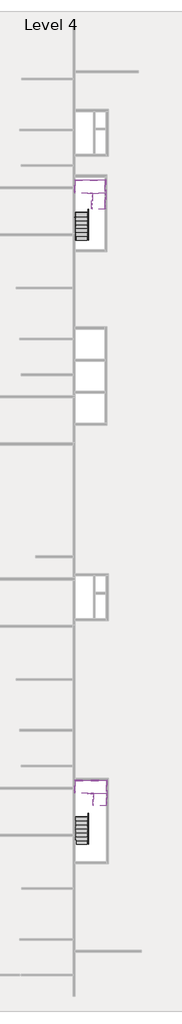
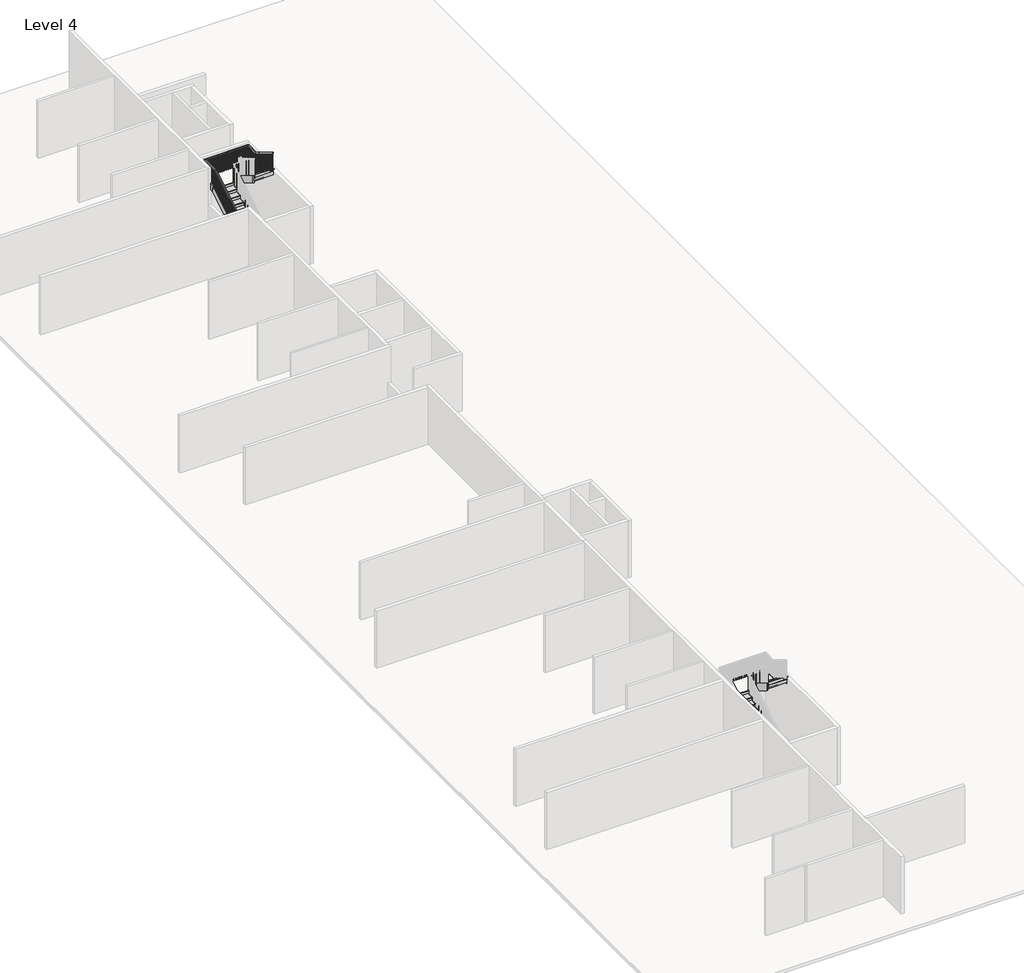
# One storey, part 8 of 8: 16 members, 4 stair flights, 2 slabs, 1 railing.
"""IFC4 building model written with IfcOpenShell, lengths in millimetres."""

from ifc_helpers import new_model, si_unit, frame, origin, place, context, project, spatial, polyline, outline, extrude, faceted_brep, transform, mapped, element, save
from components import non_monolithic_landing_46a25b39, non_monolithic_landing_d45999a6, stair_flight_ca28c9d9, stair_flight_c52ec63c, stair_flight_74cd6fce, stair_flight_e8b6355c

model = new_model("IFC4")

# Units and contexts
model_context = context("Model", 3, world=origin())
ifc_project = project(units=[si_unit("LENGTHUNIT", "METRE", prefix="MILLI")], contexts=[model_context])

# Site, building, storey
site = spatial("IfcSite", under=ifc_project)
building = spatial("IfcBuilding", under=site)
storey = spatial("IfcBuildingStorey", under=building, Name="Level 4", Elevation=34378.6172466)

# Members
placement = place(None, origin())
element("IfcMember", 1, ObjectType="Stringer - 2\" Width", at=placement, inside=storey, context=model_context, shape_type="SweptSolid", body=[
    extrude(outline(polyline([(-23154.3851539, 34378.6172466), (-23154.3851539, 34590.7317586), (-19467.0440987, 36825.4839133), (-19381.8896422, 36520.6839133), (-22916.2996422, 34378.6172466), (-23154.3851539, 34378.6172466)])), frame((-3668.2415084, 0.0, 0.0), z_axis=(1.0, 0.0, 0.0), x_axis=(0.0, 1.0, 0.0)), (0.0, 0.0, 1.0), 50.8),
])
element("IfcMember", 2, ObjectType="Stringer - 2\" Width", at=placement, inside=storey, context=model_context, shape_type="SweptSolid", body=[
    extrude(outline(polyline([(-23154.3851539, 34378.6172466), (-23154.3851539, 34590.7317586), (-19572.9851539, 36761.2772131), (-19572.9851539, 36404.8684516), (-22916.2996422, 34378.6172466), (-23154.3851539, 34378.6172466)])), frame((-2703.0415084, 0.0, 0.0), z_axis=(1.0, 0.0, 0.0), x_axis=(0.0, 1.0, 0.0)), (0.0, 0.0, 1.0), 50.8),
])
element("IfcMember", 3, ObjectType="Stringer - 2\" Width", at=placement, inside=storey, context=model_context, shape_type="SweptSolid", body=[
    extrude(outline(polyline([(-19297.9262092, 36825.4839133), (-19383.0806657, 36520.6839133), (-20360.3851539, 37112.9896637), (-20360.3851539, 37469.3984252), (-19297.9262092, 36825.4839133)])), frame((-1382.2415084, 0.0, 0.0), z_axis=(1.0, 0.0, 0.0), x_axis=(0.0, 1.0, 0.0)), (0.0, 0.0, 1.0), 50.8),
])
element("IfcMember", 4, ObjectType="Stringer - 2\" Width", at=placement, inside=storey, context=model_context, shape_type="SweptSolid", body=[
    extrude(outline(polyline([(-19522.1851539, 36961.3984252), (-19522.1851539, 36604.9896637), (-20360.3851539, 37112.9896637), (-20360.3851539, 37469.3984252), (-19522.1851539, 36961.3984252)])), frame((-2347.4415084, 0.0, 0.0), z_axis=(1.0, 0.0, 0.0), x_axis=(0.0, 1.0, 0.0)), (0.0, 0.0, 1.0), 50.8),
])
element("IfcMember", 5, ObjectType="Stringer - 2\" Width", at=placement, inside=storey, context=model_context, shape_type="Brep", body=[
    faceted_brep([(-1382.2415084, -19297.9262092, 36825.4839133), (-1331.4415084, -19297.9262092, 36825.4839133), (-1331.4415084, -18556.9851539, 36825.4839133), (-1382.2415084, -18607.7851539, 36825.4839133), (-1382.2415084, -19383.0806657, 36520.6839133), (-1382.2415084, -18607.7851539, 36520.6839133), (-1331.4415084, -19383.0806657, 36520.6839133), (-1331.4415084, -18556.9851539, 36520.6839133)], [[[0, 1, 2, 3]], [[4, 0, 3, 5]], [[6, 4, 5, 7]], [[1, 6, 7, 2]], [[1, 0, 4, 6]], [[2, 7, 5, 3]]]),
])
element("IfcMember", 6, ObjectType="Stringer - 2\" Width", at=placement, inside=storey, context=model_context, shape_type="SweptSolid", body=[
    extrude(outline(polyline([(-1331.4415084, -18556.9851539), (-1382.2415084, -18607.7851539), (-3617.4415084, -18607.7851539), (-3668.2415084, -18556.9851539), (-1331.4415084, -18556.9851539)])), frame((0.0, 0.0, 36520.6839133), z_axis=(0.0, 0.0, 1.0), x_axis=(1.0, 0.0, 0.0)), (0.0, 0.0, 1.0), 304.8),
])
element("IfcMember", 7, ObjectType="Stringer - 2\" Width", at=placement, inside=storey, context=model_context, shape_type="Brep", body=[
    faceted_brep([(-3617.4415084, -18607.7851539, 36825.4839133), (-3668.2415084, -18556.9851539, 36825.4839133), (-3668.2415084, -19467.0440987, 36825.4839133), (-3617.4415084, -19467.0440987, 36825.4839133), (-3617.4415084, -18607.7851539, 36520.6839133), (-3617.4415084, -19381.8896422, 36520.6839133), (-3668.2415084, -18556.9851539, 36520.6839133), (-3668.2415084, -19381.8896422, 36520.6839133)], [[[0, 1, 2, 3]], [[4, 0, 3, 5]], [[6, 4, 5, 7]], [[1, 6, 7, 2]], [[1, 0, 4, 6]], [[2, 7, 5, 3]]]),
])
element("IfcMember", 8, ObjectType="Stringer - 2\" Width", at=placement, inside=storey, context=model_context, shape_type="SweptSolid", body=[
    extrude(outline(polyline([(-2703.0415084, -19572.9851539), (-2703.0415084, -19522.1851539), (-2347.4415084, -19522.1851539), (-2347.4415084, -19572.9851539), (-2703.0415084, -19572.9851539)])), frame((0.0, 0.0, 36520.6839133), z_axis=(0.0, 0.0, 1.0), x_axis=(1.0, 0.0, 0.0)), (0.0, 0.0, 1.0), 304.8),
])
element("IfcMember", 9, ObjectType="Stringer - 2\" Width", at=placement, inside=storey, context=model_context, shape_type="SweptSolid", body=[
    extrude(outline(polyline([(19841.9216096, 34378.6172466), (19841.9216096, 34590.7317586), (23249.8626649, 36656.1505799), (23335.0171214, 36351.3505799), (20080.0071214, 34378.6172466), (19841.9216096, 34378.6172466)])), frame((-3668.2415084, 0.0, 0.0), z_axis=(1.0, 0.0, 0.0), x_axis=(0.0, 1.0, 0.0)), (0.0, 0.0, 1.0), 50.8),
])
element("IfcMember", 10, ObjectType="Stringer - 2\" Width", at=placement, inside=storey, context=model_context, shape_type="SweptSolid", body=[
    extrude(outline(polyline([(19841.9216096, 34378.6172466), (19841.9216096, 34590.7317586), (23143.9216096, 36591.9438798), (23143.9216096, 36235.5351183), (20080.0071214, 34378.6172466), (19841.9216096, 34378.6172466)])), frame((-2703.0415084, 0.0, 0.0), z_axis=(1.0, 0.0, 0.0), x_axis=(0.0, 1.0, 0.0)), (0.0, 0.0, 1.0), 50.8),
])
element("IfcMember", 11, ObjectType="Stringer - 2\" Width", at=placement, inside=storey, context=model_context, shape_type="SweptSolid", body=[
    extrude(outline(polyline([(23418.9805543, 36656.1505799), (23333.8260978, 36351.3505799), (22077.1216096, 37112.9896637), (22077.1216096, 37469.3984252), (23418.9805543, 36656.1505799)])), frame((-1483.8415084, 0.0, 0.0), z_axis=(1.0, 0.0, 0.0), x_axis=(0.0, 1.0, 0.0)), (0.0, 0.0, 1.0), 50.8),
])
element("IfcMember", 12, ObjectType="Stringer - 2\" Width", at=placement, inside=storey, context=model_context, shape_type="SweptSolid", body=[
    extrude(outline(polyline([(23194.7216096, 36792.0650919), (23194.7216096, 36435.6563304), (22077.1216096, 37112.9896637), (22077.1216096, 37469.3984252), (23194.7216096, 36792.0650919)])), frame((-2449.0415084, 0.0, 0.0), z_axis=(1.0, 0.0, 0.0), x_axis=(0.0, 1.0, 0.0)), (0.0, 0.0, 1.0), 50.8),
])
element("IfcMember", 13, ObjectType="Stringer - 2\" Width", at=placement, inside=storey, context=model_context, shape_type="Brep", body=[
    faceted_brep([(-1483.8415084, 23418.9805543, 36656.1505799), (-1433.0415084, 23418.9805543, 36656.1505799), (-1433.0415084, 24159.9216096, 36656.1505799), (-1483.8415084, 24109.1216096, 36656.1505799), (-1483.8415084, 23333.8260978, 36351.3505799), (-1483.8415084, 24109.1216096, 36351.3505799), (-1433.0415084, 23333.8260978, 36351.3505799), (-1433.0415084, 24159.9216096, 36351.3505799)], [[[0, 1, 2, 3]], [[4, 0, 3, 5]], [[6, 4, 5, 7]], [[1, 6, 7, 2]], [[1, 0, 4, 6]], [[2, 7, 5, 3]]]),
])
element("IfcMember", 14, ObjectType="Stringer - 2\" Width", at=placement, inside=storey, context=model_context, shape_type="SweptSolid", body=[
    extrude(outline(polyline([(-1433.0415084, 24159.9216096), (-1483.8415084, 24109.1216096), (-3617.4415084, 24109.1216096), (-3668.2415084, 24159.9216096), (-1433.0415084, 24159.9216096)])), frame((0.0, 0.0, 36351.3505799), z_axis=(0.0, 0.0, 1.0), x_axis=(1.0, 0.0, 0.0)), (0.0, 0.0, 1.0), 304.8),
])
element("IfcMember", 15, ObjectType="Stringer - 2\" Width", at=placement, inside=storey, context=model_context, shape_type="Brep", body=[
    faceted_brep([(-3617.4415084, 24109.1216096, 36656.1505799), (-3668.2415084, 24159.9216096, 36656.1505799), (-3668.2415084, 23249.8626649, 36656.1505799), (-3617.4415084, 23249.8626649, 36656.1505799), (-3617.4415084, 24109.1216096, 36351.3505799), (-3617.4415084, 23335.0171214, 36351.3505799), (-3668.2415084, 24159.9216096, 36351.3505799), (-3668.2415084, 23335.0171214, 36351.3505799)], [[[0, 1, 2, 3]], [[4, 0, 3, 5]], [[6, 4, 5, 7]], [[1, 6, 7, 2]], [[1, 0, 4, 6]], [[2, 7, 5, 3]]]),
])
element("IfcMember", 16, ObjectType="Stringer - 2\" Width", at=placement, inside=storey, context=model_context, shape_type="SweptSolid", body=[
    extrude(outline(polyline([(-2703.0415084, 23143.9216096), (-2703.0415084, 23194.7216096), (-2449.0415084, 23194.7216096), (-2449.0415084, 23143.9216096), (-2703.0415084, 23143.9216096)])), frame((0.0, 0.0, 36351.3505799), z_axis=(0.0, 0.0, 1.0), x_axis=(1.0, 0.0, 0.0)), (0.0, 0.0, 1.0), 304.8),
])

# Railing
element("IfcRailing", 17, ObjectType="Handrail - Rectangular", at=placement, inside=storey, context=model_context, shape_type="SolidModel", body=[
    faceted_brep([(-3617.4415084, 19841.9216096, 35462.3505799), (-3617.4415084, 19841.9216096, 35402.9491197), (-3566.6415084, 19841.9216096, 35402.9491197), (-3566.6415084, 19841.9216096, 35462.3505799), (-3617.4415084, 23194.7216096, 37494.3505799), (-3617.4415084, 23208.914019, 37443.5505799), (-3566.6415084, 23208.914019, 37443.5505799), (-3566.6415084, 23194.7216096, 37494.3505799), (-3617.4415084, 24109.1216096, 37494.3505799), (-3617.4415084, 24109.1216096, 37443.5505799), (-3566.6415084, 24058.3216096, 37443.5505799), (-3566.6415084, 24058.3216096, 37494.3505799), (-1483.8415084, 24109.1216096, 37494.3505799), (-1483.8415084, 24109.1216096, 37443.5505799), (-1534.6415084, 24058.3216096, 37443.5505799), (-1534.6415084, 24058.3216096, 37494.3505799), (-1483.8415084, 23474.1216096, 37494.3505799), (-1483.8415084, 23459.9292002, 37443.5505799), (-1534.6415084, 23459.9292002, 37443.5505799), (-1534.6415084, 23474.1216096, 37494.3505799), (-1483.8415084, 23194.7216096, 37663.6839133), (-1483.8415084, 23168.3918824, 37620.2398634), (-1534.6415084, 23168.3918824, 37620.2398634), (-1534.6415084, 23194.7216096, 37663.6839133), (-1483.8415084, 22077.1216096, 38341.0172466), (-1534.6415084, 22077.1216096, 38341.0172466), (-1534.6415084, 22077.1216096, 38281.6157863), (-1483.8415084, 22077.1216096, 38281.6157863)], [[[0, 1, 2, 3]], [[1, 0, 4, 5]], [[2, 1, 5, 6]], [[3, 2, 6, 7]], [[0, 3, 7, 4]], [[5, 4, 8, 9]], [[6, 5, 9, 10]], [[7, 6, 10, 11]], [[4, 7, 11, 8]], [[9, 8, 12, 13]], [[10, 9, 13, 14]], [[11, 10, 14, 15]], [[8, 11, 15, 12]], [[13, 12, 16, 17]], [[14, 13, 17, 18]], [[15, 14, 18, 19]], [[12, 15, 19, 16]], [[17, 16, 20, 21]], [[18, 17, 21, 22]], [[19, 18, 22, 23]], [[16, 19, 23, 20]], [[24, 25, 26, 27]], [[21, 20, 24, 27]], [[22, 21, 27, 26]], [[23, 22, 26, 25]], [[20, 23, 25, 24]]]),
    extrude(outline(polyline([(22188.2466096, 38214.2673015), (22188.2466096, 37257.2839133), (22169.1966096, 37257.2839133), (22169.1966096, 38225.812756), (22188.2466096, 38214.2673015)])), frame((-1518.7665084, 0.0, 0.0), z_axis=(1.0, 0.0, 0.0), x_axis=(0.0, 1.0, 0.0)), (0.0, 0.0, 1.0), 19.05),
    extrude(outline(polyline([(22289.8466096, 38152.6915439), (22289.8466096, 37257.2839133), (22270.7966096, 37257.2839133), (22270.7966096, 38164.2369985), (22289.8466096, 38152.6915439)])), frame((-1518.7665084, 0.0, 0.0), z_axis=(1.0, 0.0, 0.0), x_axis=(0.0, 1.0, 0.0)), (0.0, 0.0, 1.0), 19.05),
    extrude(outline(polyline([(22391.4466096, 38091.1157863), (22391.4466096, 37087.9505799), (22372.3966096, 37087.9505799), (22372.3966096, 38102.6612409), (22391.4466096, 38091.1157863)])), frame((-1518.7665084, 0.0, 0.0), z_axis=(1.0, 0.0, 0.0), x_axis=(0.0, 1.0, 0.0)), (0.0, 0.0, 1.0), 19.05),
    extrude(outline(polyline([(22493.0466096, 38029.5400288), (22493.0466096, 37087.9505799), (22473.9966096, 37087.9505799), (22473.9966096, 38041.0854833), (22493.0466096, 38029.5400288)])), frame((-1518.7665084, 0.0, 0.0), z_axis=(1.0, 0.0, 0.0), x_axis=(0.0, 1.0, 0.0)), (0.0, 0.0, 1.0), 19.05),
    extrude(outline(polyline([(22594.6466096, 37967.9642712), (22594.6466096, 37087.9505799), (22575.5966096, 37087.9505799), (22575.5966096, 37979.5097257), (22594.6466096, 37967.9642712)])), frame((-1518.7665084, 0.0, 0.0), z_axis=(1.0, 0.0, 0.0), x_axis=(0.0, 1.0, 0.0)), (0.0, 0.0, 1.0), 19.05),
    extrude(outline(polyline([(22696.2466096, 37906.3885136), (22696.2466096, 36918.6172466), (22677.1966096, 36918.6172466), (22677.1966096, 37917.9339682), (22696.2466096, 37906.3885136)])), frame((-1518.7665084, 0.0, 0.0), z_axis=(1.0, 0.0, 0.0), x_axis=(0.0, 1.0, 0.0)), (0.0, 0.0, 1.0), 19.05),
    extrude(outline(polyline([(22797.8466096, 37844.812756), (22797.8466096, 36918.6172466), (22778.7966096, 36918.6172466), (22778.7966096, 37856.3582106), (22797.8466096, 37844.812756)])), frame((-1518.7665084, 0.0, 0.0), z_axis=(1.0, 0.0, 0.0), x_axis=(0.0, 1.0, 0.0)), (0.0, 0.0, 1.0), 19.05),
    extrude(outline(polyline([(22899.4466096, 37783.2369985), (22899.4466096, 36918.6172466), (22880.3966096, 36918.6172466), (22880.3966096, 37794.782453), (22899.4466096, 37783.2369985)])), frame((-1518.7665084, 0.0, 0.0), z_axis=(1.0, 0.0, 0.0), x_axis=(0.0, 1.0, 0.0)), (0.0, 0.0, 1.0), 19.05),
    extrude(outline(polyline([(23001.0466096, 37721.6612409), (23001.0466096, 36749.2839133), (22981.9966096, 36749.2839133), (22981.9966096, 37733.2066954), (23001.0466096, 37721.6612409)])), frame((-1518.7665084, 0.0, 0.0), z_axis=(1.0, 0.0, 0.0), x_axis=(0.0, 1.0, 0.0)), (0.0, 0.0, 1.0), 19.05),
    extrude(outline(polyline([(23102.6466096, 37660.0854833), (23102.6466096, 36749.2839133), (23083.5966096, 36749.2839133), (23083.5966096, 37671.6309379), (23102.6466096, 37660.0854833)])), frame((-1518.7665084, 0.0, 0.0), z_axis=(1.0, 0.0, 0.0), x_axis=(0.0, 1.0, 0.0)), (0.0, 0.0, 1.0), 19.05),
    extrude(outline(polyline([(23280.4466096, 37552.3279076), (23280.4466096, 36579.9505799), (23261.3966096, 36579.9505799), (23261.3966096, 37563.8733621), (23280.4466096, 37552.3279076)])), frame((-1518.7665084, 0.0, 0.0), z_axis=(1.0, 0.0, 0.0), x_axis=(0.0, 1.0, 0.0)), (0.0, 0.0, 1.0), 19.05),
    extrude(outline(polyline([(23382.0466096, 37490.75215), (23382.0466096, 36579.9505799), (23362.9966096, 36579.9505799), (23362.9966096, 37502.2976045), (23382.0466096, 37490.75215)])), frame((-1518.7665084, 0.0, 0.0), z_axis=(1.0, 0.0, 0.0), x_axis=(0.0, 1.0, 0.0)), (0.0, 0.0, 1.0), 19.05),
    extrude(outline(polyline([(-1499.7165084, 23483.6466096), (-1499.7165084, 23464.5966096), (-1518.7665084, 23464.5966096), (-1518.7665084, 23483.6466096), (-1499.7165084, 23483.6466096)])), frame((0.0, 0.0, 36579.9505799), z_axis=(0.0, 0.0, 1.0), x_axis=(1.0, 0.0, 0.0)), (0.0, 0.0, 1.0), 863.6),
    extrude(outline(polyline([(-1499.7165084, 23585.2466096), (-1499.7165084, 23566.1966096), (-1518.7665084, 23566.1966096), (-1518.7665084, 23585.2466096), (-1499.7165084, 23585.2466096)])), frame((0.0, 0.0, 36579.9505799), z_axis=(0.0, 0.0, 1.0), x_axis=(1.0, 0.0, 0.0)), (0.0, 0.0, 1.0), 863.6),
    extrude(outline(polyline([(-1499.7165084, 23686.8466096), (-1499.7165084, 23667.7966096), (-1518.7665084, 23667.7966096), (-1518.7665084, 23686.8466096), (-1499.7165084, 23686.8466096)])), frame((0.0, 0.0, 36579.9505799), z_axis=(0.0, 0.0, 1.0), x_axis=(1.0, 0.0, 0.0)), (0.0, 0.0, 1.0), 863.6),
    extrude(outline(polyline([(-1499.7165084, 23788.4466096), (-1499.7165084, 23769.3966096), (-1518.7665084, 23769.3966096), (-1518.7665084, 23788.4466096), (-1499.7165084, 23788.4466096)])), frame((0.0, 0.0, 36579.9505799), z_axis=(0.0, 0.0, 1.0), x_axis=(1.0, 0.0, 0.0)), (0.0, 0.0, 1.0), 863.6),
    extrude(outline(polyline([(-1499.7165084, 23890.0466096), (-1499.7165084, 23870.9966096), (-1518.7665084, 23870.9966096), (-1518.7665084, 23890.0466096), (-1499.7165084, 23890.0466096)])), frame((0.0, 0.0, 36579.9505799), z_axis=(0.0, 0.0, 1.0), x_axis=(1.0, 0.0, 0.0)), (0.0, 0.0, 1.0), 863.6),
    extrude(outline(polyline([(-1499.7165084, 23991.6466096), (-1499.7165084, 23972.5966096), (-1518.7665084, 23972.5966096), (-1518.7665084, 23991.6466096), (-1499.7165084, 23991.6466096)])), frame((0.0, 0.0, 36579.9505799), z_axis=(0.0, 0.0, 1.0), x_axis=(1.0, 0.0, 0.0)), (0.0, 0.0, 1.0), 863.6),
    extrude(outline(polyline([(-1569.5665084, 24093.2466096), (-1550.5165084, 24093.2466096), (-1550.5165084, 24074.1966096), (-1569.5665084, 24074.1966096), (-1569.5665084, 24093.2466096)])), frame((0.0, 0.0, 36579.9505799), z_axis=(0.0, 0.0, 1.0), x_axis=(1.0, 0.0, 0.0)), (0.0, 0.0, 1.0), 863.6),
    extrude(outline(polyline([(-1671.1665084, 24093.2466096), (-1652.1165084, 24093.2466096), (-1652.1165084, 24074.1966096), (-1671.1665084, 24074.1966096), (-1671.1665084, 24093.2466096)])), frame((0.0, 0.0, 36579.9505799), z_axis=(0.0, 0.0, 1.0), x_axis=(1.0, 0.0, 0.0)), (0.0, 0.0, 1.0), 863.6),
    extrude(outline(polyline([(-1772.7665084, 24093.2466096), (-1753.7165084, 24093.2466096), (-1753.7165084, 24074.1966096), (-1772.7665084, 24074.1966096), (-1772.7665084, 24093.2466096)])), frame((0.0, 0.0, 36579.9505799), z_axis=(0.0, 0.0, 1.0), x_axis=(1.0, 0.0, 0.0)), (0.0, 0.0, 1.0), 863.6),
    extrude(outline(polyline([(-1874.3665084, 24093.2466096), (-1855.3165084, 24093.2466096), (-1855.3165084, 24074.1966096), (-1874.3665084, 24074.1966096), (-1874.3665084, 24093.2466096)])), frame((0.0, 0.0, 36579.9505799), z_axis=(0.0, 0.0, 1.0), x_axis=(1.0, 0.0, 0.0)), (0.0, 0.0, 1.0), 863.6),
    extrude(outline(polyline([(-1975.9665084, 24093.2466096), (-1956.9165084, 24093.2466096), (-1956.9165084, 24074.1966096), (-1975.9665084, 24074.1966096), (-1975.9665084, 24093.2466096)])), frame((0.0, 0.0, 36579.9505799), z_axis=(0.0, 0.0, 1.0), x_axis=(1.0, 0.0, 0.0)), (0.0, 0.0, 1.0), 863.6),
    extrude(outline(polyline([(-2077.5665084, 24093.2466096), (-2058.5165084, 24093.2466096), (-2058.5165084, 24074.1966096), (-2077.5665084, 24074.1966096), (-2077.5665084, 24093.2466096)])), frame((0.0, 0.0, 36579.9505799), z_axis=(0.0, 0.0, 1.0), x_axis=(1.0, 0.0, 0.0)), (0.0, 0.0, 1.0), 863.6),
    extrude(outline(polyline([(-2179.1665084, 24093.2466096), (-2160.1165084, 24093.2466096), (-2160.1165084, 24074.1966096), (-2179.1665084, 24074.1966096), (-2179.1665084, 24093.2466096)])), frame((0.0, 0.0, 36579.9505799), z_axis=(0.0, 0.0, 1.0), x_axis=(1.0, 0.0, 0.0)), (0.0, 0.0, 1.0), 863.6),
    extrude(outline(polyline([(-2280.7665084, 24093.2466096), (-2261.7165084, 24093.2466096), (-2261.7165084, 24074.1966096), (-2280.7665084, 24074.1966096), (-2280.7665084, 24093.2466096)])), frame((0.0, 0.0, 36579.9505799), z_axis=(0.0, 0.0, 1.0), x_axis=(1.0, 0.0, 0.0)), (0.0, 0.0, 1.0), 863.6),
    extrude(outline(polyline([(-2382.3665084, 24093.2466096), (-2363.3165084, 24093.2466096), (-2363.3165084, 24074.1966096), (-2382.3665084, 24074.1966096), (-2382.3665084, 24093.2466096)])), frame((0.0, 0.0, 36579.9505799), z_axis=(0.0, 0.0, 1.0), x_axis=(1.0, 0.0, 0.0)), (0.0, 0.0, 1.0), 863.6),
    extrude(outline(polyline([(-2483.9665084, 24093.2466096), (-2464.9165084, 24093.2466096), (-2464.9165084, 24074.1966096), (-2483.9665084, 24074.1966096), (-2483.9665084, 24093.2466096)])), frame((0.0, 0.0, 36579.9505799), z_axis=(0.0, 0.0, 1.0), x_axis=(1.0, 0.0, 0.0)), (0.0, 0.0, 1.0), 863.6),
    extrude(outline(polyline([(-2585.5665084, 24093.2466096), (-2566.5165084, 24093.2466096), (-2566.5165084, 24074.1966096), (-2585.5665084, 24074.1966096), (-2585.5665084, 24093.2466096)])), frame((0.0, 0.0, 36579.9505799), z_axis=(0.0, 0.0, 1.0), x_axis=(1.0, 0.0, 0.0)), (0.0, 0.0, 1.0), 863.6),
    extrude(outline(polyline([(-2687.1665084, 24093.2466096), (-2668.1165084, 24093.2466096), (-2668.1165084, 24074.1966096), (-2687.1665084, 24074.1966096), (-2687.1665084, 24093.2466096)])), frame((0.0, 0.0, 36579.9505799), z_axis=(0.0, 0.0, 1.0), x_axis=(1.0, 0.0, 0.0)), (0.0, 0.0, 1.0), 863.6),
    extrude(outline(polyline([(-2788.7665084, 24093.2466096), (-2769.7165084, 24093.2466096), (-2769.7165084, 24074.1966096), (-2788.7665084, 24074.1966096), (-2788.7665084, 24093.2466096)])), frame((0.0, 0.0, 36579.9505799), z_axis=(0.0, 0.0, 1.0), x_axis=(1.0, 0.0, 0.0)), (0.0, 0.0, 1.0), 863.6),
    extrude(outline(polyline([(-2890.3665084, 24093.2466096), (-2871.3165084, 24093.2466096), (-2871.3165084, 24074.1966096), (-2890.3665084, 24074.1966096), (-2890.3665084, 24093.2466096)])), frame((0.0, 0.0, 36579.9505799), z_axis=(0.0, 0.0, 1.0), x_axis=(1.0, 0.0, 0.0)), (0.0, 0.0, 1.0), 863.6),
    extrude(outline(polyline([(-2991.9665084, 24093.2466096), (-2972.9165084, 24093.2466096), (-2972.9165084, 24074.1966096), (-2991.9665084, 24074.1966096), (-2991.9665084, 24093.2466096)])), frame((0.0, 0.0, 36579.9505799), z_axis=(0.0, 0.0, 1.0), x_axis=(1.0, 0.0, 0.0)), (0.0, 0.0, 1.0), 863.6),
    extrude(outline(polyline([(-3093.5665084, 24093.2466096), (-3074.5165084, 24093.2466096), (-3074.5165084, 24074.1966096), (-3093.5665084, 24074.1966096), (-3093.5665084, 24093.2466096)])), frame((0.0, 0.0, 36579.9505799), z_axis=(0.0, 0.0, 1.0), x_axis=(1.0, 0.0, 0.0)), (0.0, 0.0, 1.0), 863.6),
    extrude(outline(polyline([(-3195.1665084, 24093.2466096), (-3176.1165084, 24093.2466096), (-3176.1165084, 24074.1966096), (-3195.1665084, 24074.1966096), (-3195.1665084, 24093.2466096)])), frame((0.0, 0.0, 36579.9505799), z_axis=(0.0, 0.0, 1.0), x_axis=(1.0, 0.0, 0.0)), (0.0, 0.0, 1.0), 863.6),
    extrude(outline(polyline([(-3296.7665084, 24093.2466096), (-3277.7165084, 24093.2466096), (-3277.7165084, 24074.1966096), (-3296.7665084, 24074.1966096), (-3296.7665084, 24093.2466096)])), frame((0.0, 0.0, 36579.9505799), z_axis=(0.0, 0.0, 1.0), x_axis=(1.0, 0.0, 0.0)), (0.0, 0.0, 1.0), 863.6),
    extrude(outline(polyline([(-3398.3665084, 24093.2466096), (-3379.3165084, 24093.2466096), (-3379.3165084, 24074.1966096), (-3398.3665084, 24074.1966096), (-3398.3665084, 24093.2466096)])), frame((0.0, 0.0, 36579.9505799), z_axis=(0.0, 0.0, 1.0), x_axis=(1.0, 0.0, 0.0)), (0.0, 0.0, 1.0), 863.6),
    extrude(outline(polyline([(-3499.9665084, 24093.2466096), (-3480.9165084, 24093.2466096), (-3480.9165084, 24074.1966096), (-3499.9665084, 24074.1966096), (-3499.9665084, 24093.2466096)])), frame((0.0, 0.0, 36579.9505799), z_axis=(0.0, 0.0, 1.0), x_axis=(1.0, 0.0, 0.0)), (0.0, 0.0, 1.0), 863.6),
    extrude(outline(polyline([(-3601.5665084, 23997.9966096), (-3601.5665084, 24017.0466096), (-3582.5165084, 24017.0466096), (-3582.5165084, 23997.9966096), (-3601.5665084, 23997.9966096)])), frame((0.0, 0.0, 36579.9505799), z_axis=(0.0, 0.0, 1.0), x_axis=(1.0, 0.0, 0.0)), (0.0, 0.0, 1.0), 863.6),
    extrude(outline(polyline([(-3601.5665084, 23896.3966096), (-3601.5665084, 23915.4466096), (-3582.5165084, 23915.4466096), (-3582.5165084, 23896.3966096), (-3601.5665084, 23896.3966096)])), frame((0.0, 0.0, 36579.9505799), z_axis=(0.0, 0.0, 1.0), x_axis=(1.0, 0.0, 0.0)), (0.0, 0.0, 1.0), 863.6),
    extrude(outline(polyline([(-3601.5665084, 23794.7966096), (-3601.5665084, 23813.8466096), (-3582.5165084, 23813.8466096), (-3582.5165084, 23794.7966096), (-3601.5665084, 23794.7966096)])), frame((0.0, 0.0, 36579.9505799), z_axis=(0.0, 0.0, 1.0), x_axis=(1.0, 0.0, 0.0)), (0.0, 0.0, 1.0), 863.6),
    extrude(outline(polyline([(-3601.5665084, 23693.1966096), (-3601.5665084, 23712.2466096), (-3582.5165084, 23712.2466096), (-3582.5165084, 23693.1966096), (-3601.5665084, 23693.1966096)])), frame((0.0, 0.0, 36579.9505799), z_axis=(0.0, 0.0, 1.0), x_axis=(1.0, 0.0, 0.0)), (0.0, 0.0, 1.0), 863.6),
    extrude(outline(polyline([(-3601.5665084, 23591.5966096), (-3601.5665084, 23610.6466096), (-3582.5165084, 23610.6466096), (-3582.5165084, 23591.5966096), (-3601.5665084, 23591.5966096)])), frame((0.0, 0.0, 36579.9505799), z_axis=(0.0, 0.0, 1.0), x_axis=(1.0, 0.0, 0.0)), (0.0, 0.0, 1.0), 863.6),
    extrude(outline(polyline([(-3601.5665084, 23489.9966096), (-3601.5665084, 23509.0466096), (-3582.5165084, 23509.0466096), (-3582.5165084, 23489.9966096), (-3601.5665084, 23489.9966096)])), frame((0.0, 0.0, 36579.9505799), z_axis=(0.0, 0.0, 1.0), x_axis=(1.0, 0.0, 0.0)), (0.0, 0.0, 1.0), 863.6),
    extrude(outline(polyline([(-3601.5665084, 23388.3966096), (-3601.5665084, 23407.4466096), (-3582.5165084, 23407.4466096), (-3582.5165084, 23388.3966096), (-3601.5665084, 23388.3966096)])), frame((0.0, 0.0, 36579.9505799), z_axis=(0.0, 0.0, 1.0), x_axis=(1.0, 0.0, 0.0)), (0.0, 0.0, 1.0), 863.6),
    extrude(outline(polyline([(-3601.5665084, 23286.7966096), (-3601.5665084, 23305.8466096), (-3582.5165084, 23305.8466096), (-3582.5165084, 23286.7966096), (-3601.5665084, 23286.7966096)])), frame((0.0, 0.0, 36579.9505799), z_axis=(0.0, 0.0, 1.0), x_axis=(1.0, 0.0, 0.0)), (0.0, 0.0, 1.0), 863.6),
    extrude(outline(polyline([(23102.6466096, 37379.1460894), (23102.6466096, 36410.6172466), (23083.5966096, 36410.6172466), (23083.5966096, 37367.6006348), (23102.6466096, 37379.1460894)])), frame((-3601.5665084, 0.0, 0.0), z_axis=(1.0, 0.0, 0.0), x_axis=(0.0, 1.0, 0.0)), (0.0, 0.0, 1.0), 19.05),
    extrude(outline(polyline([(23001.0466096, 37317.5703318), (23001.0466096, 36410.6172466), (22981.9966096, 36410.6172466), (22981.9966096, 37306.0248773), (23001.0466096, 37317.5703318)])), frame((-3601.5665084, 0.0, 0.0), z_axis=(1.0, 0.0, 0.0), x_axis=(0.0, 1.0, 0.0)), (0.0, 0.0, 1.0), 19.05),
    extrude(outline(polyline([(22899.4466096, 37255.9945742), (22899.4466096, 36241.2839133), (22880.3966096, 36241.2839133), (22880.3966096, 37244.4491197), (22899.4466096, 37255.9945742)])), frame((-3601.5665084, 0.0, 0.0), z_axis=(1.0, 0.0, 0.0), x_axis=(0.0, 1.0, 0.0)), (0.0, 0.0, 1.0), 19.05),
    extrude(outline(polyline([(22797.8466096, 37194.4188166), (22797.8466096, 36241.2839133), (22778.7966096, 36241.2839133), (22778.7966096, 37182.8733621), (22797.8466096, 37194.4188166)])), frame((-3601.5665084, 0.0, 0.0), z_axis=(1.0, 0.0, 0.0), x_axis=(0.0, 1.0, 0.0)), (0.0, 0.0, 1.0), 19.05),
    extrude(outline(polyline([(22696.2466096, 37132.8430591), (22696.2466096, 36241.2839133), (22677.1966096, 36241.2839133), (22677.1966096, 37121.2976045), (22696.2466096, 37132.8430591)])), frame((-3601.5665084, 0.0, 0.0), z_axis=(1.0, 0.0, 0.0), x_axis=(0.0, 1.0, 0.0)), (0.0, 0.0, 1.0), 19.05),
    extrude(outline(polyline([(22594.6466096, 37071.2673015), (22594.6466096, 36071.9505799), (22575.5966096, 36071.9505799), (22575.5966096, 37059.721847), (22594.6466096, 37071.2673015)])), frame((-3601.5665084, 0.0, 0.0), z_axis=(1.0, 0.0, 0.0), x_axis=(0.0, 1.0, 0.0)), (0.0, 0.0, 1.0), 19.05),
    extrude(outline(polyline([(22493.0466096, 37009.6915439), (22493.0466096, 36071.9505799), (22473.9966096, 36071.9505799), (22473.9966096, 36998.1460894), (22493.0466096, 37009.6915439)])), frame((-3601.5665084, 0.0, 0.0), z_axis=(1.0, 0.0, 0.0), x_axis=(0.0, 1.0, 0.0)), (0.0, 0.0, 1.0), 19.05),
    extrude(outline(polyline([(22391.4466096, 36948.1157863), (22391.4466096, 36071.9505799), (22372.3966096, 36071.9505799), (22372.3966096, 36936.5703318), (22391.4466096, 36948.1157863)])), frame((-3601.5665084, 0.0, 0.0), z_axis=(1.0, 0.0, 0.0), x_axis=(0.0, 1.0, 0.0)), (0.0, 0.0, 1.0), 19.05),
    extrude(outline(polyline([(22289.8466096, 36886.5400288), (22289.8466096, 35902.6172466), (22270.7966096, 35902.6172466), (22270.7966096, 36874.9945742), (22289.8466096, 36886.5400288)])), frame((-3601.5665084, 0.0, 0.0), z_axis=(1.0, 0.0, 0.0), x_axis=(0.0, 1.0, 0.0)), (0.0, 0.0, 1.0), 19.05),
    extrude(outline(polyline([(22188.2466096, 36824.9642712), (22188.2466096, 35902.6172466), (22169.1966096, 35902.6172466), (22169.1966096, 36813.4188166), (22188.2466096, 36824.9642712)])), frame((-3601.5665084, 0.0, 0.0), z_axis=(1.0, 0.0, 0.0), x_axis=(0.0, 1.0, 0.0)), (0.0, 0.0, 1.0), 19.05),
    extrude(outline(polyline([(22086.6466096, 36763.3885136), (22086.6466096, 35902.6172466), (22067.5966096, 35902.6172466), (22067.5966096, 36751.8430591), (22086.6466096, 36763.3885136)])), frame((-3601.5665084, 0.0, 0.0), z_axis=(1.0, 0.0, 0.0), x_axis=(0.0, 1.0, 0.0)), (0.0, 0.0, 1.0), 19.05),
    extrude(outline(polyline([(21985.0466096, 36701.812756), (21985.0466096, 35733.2839133), (21965.9966096, 35733.2839133), (21965.9966096, 36690.2673015), (21985.0466096, 36701.812756)])), frame((-3601.5665084, 0.0, 0.0), z_axis=(1.0, 0.0, 0.0), x_axis=(0.0, 1.0, 0.0)), (0.0, 0.0, 1.0), 19.05),
    extrude(outline(polyline([(21883.4466096, 36640.2369985), (21883.4466096, 35733.2839133), (21864.3966096, 35733.2839133), (21864.3966096, 36628.6915439), (21883.4466096, 36640.2369985)])), frame((-3601.5665084, 0.0, 0.0), z_axis=(1.0, 0.0, 0.0), x_axis=(0.0, 1.0, 0.0)), (0.0, 0.0, 1.0), 19.05),
    extrude(outline(polyline([(21781.8466096, 36578.6612409), (21781.8466096, 35563.9505799), (21762.7966096, 35563.9505799), (21762.7966096, 36567.1157863), (21781.8466096, 36578.6612409)])), frame((-3601.5665084, 0.0, 0.0), z_axis=(1.0, 0.0, 0.0), x_axis=(0.0, 1.0, 0.0)), (0.0, 0.0, 1.0), 19.05),
    extrude(outline(polyline([(21680.2466096, 36517.0854833), (21680.2466096, 35563.9505799), (21661.1966096, 35563.9505799), (21661.1966096, 36505.5400288), (21680.2466096, 36517.0854833)])), frame((-3601.5665084, 0.0, 0.0), z_axis=(1.0, 0.0, 0.0), x_axis=(0.0, 1.0, 0.0)), (0.0, 0.0, 1.0), 19.05),
    extrude(outline(polyline([(21578.6466096, 36455.5097257), (21578.6466096, 35563.9505799), (21559.5966096, 35563.9505799), (21559.5966096, 36443.9642712), (21578.6466096, 36455.5097257)])), frame((-3601.5665084, 0.0, 0.0), z_axis=(1.0, 0.0, 0.0), x_axis=(0.0, 1.0, 0.0)), (0.0, 0.0, 1.0), 19.05),
    extrude(outline(polyline([(21477.0466096, 36393.9339682), (21477.0466096, 35394.6172466), (21457.9966096, 35394.6172466), (21457.9966096, 36382.3885136), (21477.0466096, 36393.9339682)])), frame((-3601.5665084, 0.0, 0.0), z_axis=(1.0, 0.0, 0.0), x_axis=(0.0, 1.0, 0.0)), (0.0, 0.0, 1.0), 19.05),
    extrude(outline(polyline([(21375.4466096, 36332.3582106), (21375.4466096, 35394.6172466), (21356.3966096, 35394.6172466), (21356.3966096, 36320.812756), (21375.4466096, 36332.3582106)])), frame((-3601.5665084, 0.0, 0.0), z_axis=(1.0, 0.0, 0.0), x_axis=(0.0, 1.0, 0.0)), (0.0, 0.0, 1.0), 19.05),
    extrude(outline(polyline([(21273.8466096, 36270.782453), (21273.8466096, 35394.6172466), (21254.7966096, 35394.6172466), (21254.7966096, 36259.2369985), (21273.8466096, 36270.782453)])), frame((-3601.5665084, 0.0, 0.0), z_axis=(1.0, 0.0, 0.0), x_axis=(0.0, 1.0, 0.0)), (0.0, 0.0, 1.0), 19.05),
    extrude(outline(polyline([(21172.2466096, 36209.2066954), (21172.2466096, 35225.2839133), (21153.1966096, 35225.2839133), (21153.1966096, 36197.6612409), (21172.2466096, 36209.2066954)])), frame((-3601.5665084, 0.0, 0.0), z_axis=(1.0, 0.0, 0.0), x_axis=(0.0, 1.0, 0.0)), (0.0, 0.0, 1.0), 19.05),
    extrude(outline(polyline([(21070.6466096, 36147.6309379), (21070.6466096, 35225.2839133), (21051.5966096, 35225.2839133), (21051.5966096, 36136.0854833), (21070.6466096, 36147.6309379)])), frame((-3601.5665084, 0.0, 0.0), z_axis=(1.0, 0.0, 0.0), x_axis=(0.0, 1.0, 0.0)), (0.0, 0.0, 1.0), 19.05),
    extrude(outline(polyline([(20969.0466096, 36086.0551803), (20969.0466096, 35225.2839133), (20949.9966096, 35225.2839133), (20949.9966096, 36074.5097257), (20969.0466096, 36086.0551803)])), frame((-3601.5665084, 0.0, 0.0), z_axis=(1.0, 0.0, 0.0), x_axis=(0.0, 1.0, 0.0)), (0.0, 0.0, 1.0), 19.05),
    extrude(outline(polyline([(20867.4466096, 36024.4794227), (20867.4466096, 35055.9505799), (20848.3966096, 35055.9505799), (20848.3966096, 36012.9339682), (20867.4466096, 36024.4794227)])), frame((-3601.5665084, 0.0, 0.0), z_axis=(1.0, 0.0, 0.0), x_axis=(0.0, 1.0, 0.0)), (0.0, 0.0, 1.0), 19.05),
    extrude(outline(polyline([(20765.8466096, 35962.9036651), (20765.8466096, 35055.9505799), (20746.7966096, 35055.9505799), (20746.7966096, 35951.3582106), (20765.8466096, 35962.9036651)])), frame((-3601.5665084, 0.0, 0.0), z_axis=(1.0, 0.0, 0.0), x_axis=(0.0, 1.0, 0.0)), (0.0, 0.0, 1.0), 19.05),
    extrude(outline(polyline([(20664.2466096, 35901.3279076), (20664.2466096, 34886.6172466), (20645.1966096, 34886.6172466), (20645.1966096, 35889.782453), (20664.2466096, 35901.3279076)])), frame((-3601.5665084, 0.0, 0.0), z_axis=(1.0, 0.0, 0.0), x_axis=(0.0, 1.0, 0.0)), (0.0, 0.0, 1.0), 19.05),
    extrude(outline(polyline([(20562.6466096, 35839.75215), (20562.6466096, 34886.6172466), (20543.5966096, 34886.6172466), (20543.5966096, 35828.2066954), (20562.6466096, 35839.75215)])), frame((-3601.5665084, 0.0, 0.0), z_axis=(1.0, 0.0, 0.0), x_axis=(0.0, 1.0, 0.0)), (0.0, 0.0, 1.0), 19.05),
    extrude(outline(polyline([(20461.0466096, 35778.1763924), (20461.0466096, 34886.6172466), (20441.9966096, 34886.6172466), (20441.9966096, 35766.6309379), (20461.0466096, 35778.1763924)])), frame((-3601.5665084, 0.0, 0.0), z_axis=(1.0, 0.0, 0.0), x_axis=(0.0, 1.0, 0.0)), (0.0, 0.0, 1.0), 19.05),
    extrude(outline(polyline([(20359.4466096, 35716.6006348), (20359.4466096, 34717.2839133), (20340.3966096, 34717.2839133), (20340.3966096, 35705.0551803), (20359.4466096, 35716.6006348)])), frame((-3601.5665084, 0.0, 0.0), z_axis=(1.0, 0.0, 0.0), x_axis=(0.0, 1.0, 0.0)), (0.0, 0.0, 1.0), 19.05),
    extrude(outline(polyline([(20257.8466096, 35655.0248773), (20257.8466096, 34717.2839133), (20238.7966096, 34717.2839133), (20238.7966096, 35643.4794227), (20257.8466096, 35655.0248773)])), frame((-3601.5665084, 0.0, 0.0), z_axis=(1.0, 0.0, 0.0), x_axis=(0.0, 1.0, 0.0)), (0.0, 0.0, 1.0), 19.05),
    extrude(outline(polyline([(20156.2466096, 35593.4491197), (20156.2466096, 34717.2839133), (20137.1966096, 34717.2839133), (20137.1966096, 35581.9036651), (20156.2466096, 35593.4491197)])), frame((-3601.5665084, 0.0, 0.0), z_axis=(1.0, 0.0, 0.0), x_axis=(0.0, 1.0, 0.0)), (0.0, 0.0, 1.0), 19.05),
    extrude(outline(polyline([(20054.6466096, 35531.8733621), (20054.6466096, 34547.9505799), (20035.5966096, 34547.9505799), (20035.5966096, 35520.3279076), (20054.6466096, 35531.8733621)])), frame((-3601.5665084, 0.0, 0.0), z_axis=(1.0, 0.0, 0.0), x_axis=(0.0, 1.0, 0.0)), (0.0, 0.0, 1.0), 19.05),
    extrude(outline(polyline([(19953.0466096, 35470.2976045), (19953.0466096, 34547.9505799), (19933.9966096, 34547.9505799), (19933.9966096, 35458.75215), (19953.0466096, 35470.2976045)])), frame((-3601.5665084, 0.0, 0.0), z_axis=(1.0, 0.0, 0.0), x_axis=(0.0, 1.0, 0.0)), (0.0, 0.0, 1.0), 19.05),
    extrude(outline(polyline([(23204.2466096, 37598.5097257), (23204.2466096, 36579.9505799), (23185.1966096, 36579.9505799), (23185.1966096, 37610.0551803), (23204.2466096, 37598.5097257)])), frame((-1518.7665084, 0.0, 0.0), z_axis=(1.0, 0.0, 0.0), x_axis=(0.0, 1.0, 0.0)), (0.0, 0.0, 1.0), 19.05),
    extrude(outline(polyline([(-1518.7665084, 24093.2466096), (-1499.7165084, 24093.2466096), (-1499.7165084, 24074.1966096), (-1518.7665084, 24074.1966096), (-1518.7665084, 24093.2466096)])), frame((0.0, 0.0, 36579.9505799), z_axis=(0.0, 0.0, 1.0), x_axis=(1.0, 0.0, 0.0)), (0.0, 0.0, 1.0), 863.6),
    extrude(outline(polyline([(-3601.5665084, 24074.1966096), (-3601.5665084, 24093.2466096), (-3582.5165084, 24093.2466096), (-3582.5165084, 24074.1966096), (-3601.5665084, 24074.1966096)])), frame((0.0, 0.0, 36579.9505799), z_axis=(0.0, 0.0, 1.0), x_axis=(1.0, 0.0, 0.0)), (0.0, 0.0, 1.0), 863.6),
    extrude(outline(polyline([(23204.2466096, 37440.721847), (23204.2466096, 36579.9505799), (23185.1966096, 36579.9505799), (23185.1966096, 37429.1763924), (23204.2466096, 37440.721847)])), frame((-3601.5665084, 0.0, 0.0), z_axis=(1.0, 0.0, 0.0), x_axis=(0.0, 1.0, 0.0)), (0.0, 0.0, 1.0), 19.05),
    extrude(outline(polyline([(22096.1716096, 38270.0703318), (22096.1716096, 37257.2839133), (22077.1216096, 37257.2839133), (22077.1216096, 38281.6157863), (22096.1716096, 38270.0703318)])), frame((-1518.7665084, 0.0, 0.0), z_axis=(1.0, 0.0, 0.0), x_axis=(0.0, 1.0, 0.0)), (0.0, 0.0, 1.0), 19.05),
    extrude(outline(polyline([(19860.9716096, 35414.4945742), (19860.9716096, 34547.9505799), (19841.9216096, 34547.9505799), (19841.9216096, 35402.9491197), (19860.9716096, 35414.4945742)])), frame((-3601.5665084, 0.0, 0.0), z_axis=(1.0, 0.0, 0.0), x_axis=(0.0, 1.0, 0.0)), (0.0, 0.0, 1.0), 19.05),
])

# Slabs
non_monolithic_landing_shape = non_monolithic_landing_46a25b39(model_context)
element("IfcSlab", 18, ObjectType="Non-Monolithic Landing", at=placement, inside=storey, context=model_context, shape_type="MappedRepresentation", body=[
    mapped(non_monolithic_landing_shape, transform((0.0, 0.0, 0.0), x_axis=(1.0, 0.0, 0.0), y_axis=(0.0, 1.0, 0.0), z_axis=(0.0, 0.0, 1.0))),
])
non_monolithic_landing_2_shape = non_monolithic_landing_d45999a6(model_context)
element("IfcSlab", 19, ObjectType="Non-Monolithic Landing", at=placement, inside=storey, context=model_context, shape_type="MappedRepresentation", body=[
    mapped(non_monolithic_landing_2_shape, transform((0.0, 0.0, 0.0), x_axis=(1.0, 0.0, 0.0), y_axis=(0.0, 1.0, 0.0), z_axis=(0.0, 0.0, 1.0))),
])

# Stair flights
stair_flight_shape = stair_flight_ca28c9d9(model_context)
element("IfcStairFlight", 20, ObjectType="2\" Tread 1\" Nosing 1/4\" Riser", at=placement, inside=storey, context=model_context, shape_type="MappedRepresentation", body=[
    mapped(stair_flight_shape, transform((0.0, 0.0, 0.0), x_axis=(1.0, 0.0, 0.0), y_axis=(0.0, 1.0, 0.0), z_axis=(0.0, 0.0, 1.0))),
])
stair_flight_2_shape = stair_flight_c52ec63c(model_context)
element("IfcStairFlight", 21, ObjectType="2\" Tread 1\" Nosing 1/4\" Riser", at=placement, inside=storey, context=model_context, shape_type="MappedRepresentation", body=[
    mapped(stair_flight_2_shape, transform((0.0, 0.0, 0.0), x_axis=(1.0, 0.0, 0.0), y_axis=(0.0, 1.0, 0.0), z_axis=(0.0, 0.0, 1.0))),
])
stair_flight_3_shape = stair_flight_74cd6fce(model_context)
element("IfcStairFlight", 22, ObjectType="2\" Tread 1\" Nosing 1/4\" Riser", at=placement, inside=storey, context=model_context, shape_type="MappedRepresentation", body=[
    mapped(stair_flight_3_shape, transform((0.0, 0.0, 0.0), x_axis=(1.0, 0.0, 0.0), y_axis=(0.0, 1.0, 0.0), z_axis=(0.0, 0.0, 1.0))),
])
stair_flight_4_shape = stair_flight_e8b6355c(model_context)
element("IfcStairFlight", 23, ObjectType="2\" Tread 1\" Nosing 1/4\" Riser", at=placement, inside=storey, context=model_context, shape_type="MappedRepresentation", body=[
    mapped(stair_flight_4_shape, transform((0.0, 0.0, 0.0), x_axis=(1.0, 0.0, 0.0), y_axis=(0.0, 1.0, 0.0), z_axis=(0.0, 0.0, 1.0))),
])

save(model, "model.ifc")

# Revit data of these elements
# Type "Handrail - Rectangular"
#   Assembly Code = "C2010400"
#   built-in parameter 1008612 = 0.0416667 (stored number, unit not read)
#   built-in parameter 1008611 = 0.0416667 (stored number, unit not read)
#   built-in parameter 1008609 = 0.333333 (stored number, unit not read)
#   built-in parameter 1008604 = 0.166667 (stored number, unit not read)
#   built-in parameter 1008603 = 0.166667 (stored number, unit not read)
#   Railing Height = 3' - 0"
#   built-in parameter 1008630 = 2
#   built-in parameter 1008610 = 2
#   built-in parameter 1008618 = Baluster - Square : 3/4"
# Elements 1, 2, 3, 4, 5, 6, 7, 8, 9, 10, 11, 12, 13, 14, 15, 16 (IfcMember, "Stringer - 2\" Width")
#   Phase Created = New Construction
# Element 17 (IfcRailing, "Handrail - Rectangular")
#   Phase Created = New Construction
# Elements 18, 19 (IfcSlab, "Non-Monolithic Landing")
#   Phase Created = New Construction
# Elements 20, 21, 22, 23 (IfcStairFlight, "2\" Tread 1\" Nosing 1/4\" Riser")
#   Phase Created = New Construction
